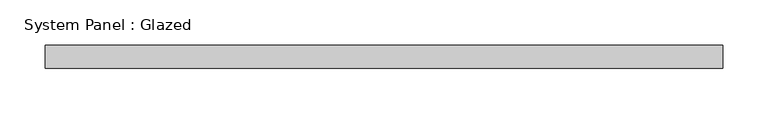
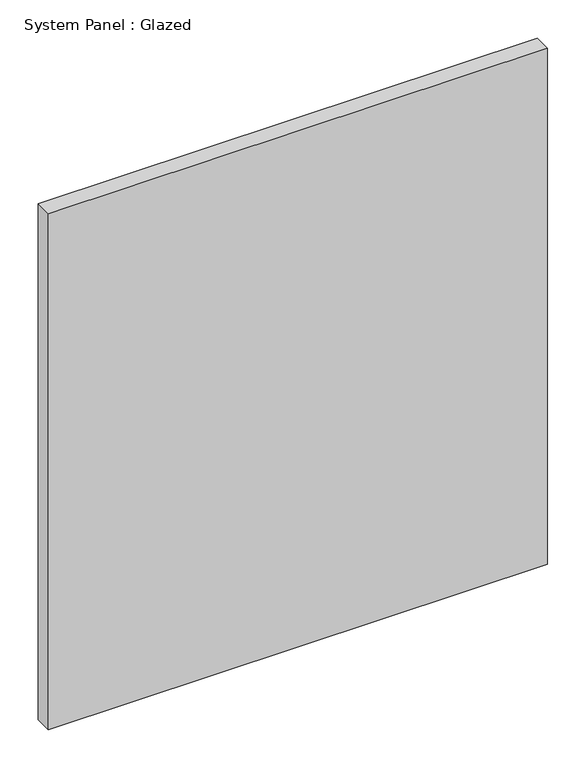
"""IFC4 building model written with IfcOpenShell, lengths in millimetres: plate geometry, System Panel : Glazed."""

from ifc_helpers import new_model, si_unit, origin, origin_with_axes, place, context, project, spatial, polyline, outline, extrude, source, transform, mapped, element, save


def system_panel_glazed_3c8ea7cb(model_context):
    return source(origin(), model_context, "Body", "SweptSolid", [
        extrude(outline(polyline([(374.65, 19.05), (-374.65, 19.05), (-374.65, 44.45), (374.65, 44.45), (374.65, 19.05)])), origin_with_axes(), (0.0, 0.0, 1.0), 818.549557),
    ])


if __name__ == "__main__":
    model = new_model("IFC4")
    model_context = context("Model", 3, world=origin())
    ifc_project = project(units=[si_unit("LENGTHUNIT", "METRE", prefix="MILLI")], contexts=[model_context])
    site = spatial("IfcSite", under=ifc_project)
    building = spatial("IfcBuilding", under=site)
    placement = place(None, origin())
    system_panel_glazed_shape = system_panel_glazed_3c8ea7cb(model_context)
    element("IfcPlate", 1, ObjectType="System Panel : Glazed", at=placement, inside=building, context=model_context, shape_type="MappedRepresentation", body=[
        mapped(system_panel_glazed_shape, transform((0.0, 0.0, 0.0), x_axis=(1.0, 0.0, 0.0), y_axis=(0.0, 1.0, 0.0), z_axis=(0.0, 0.0, 1.0))),
    ])
    save(model, "model.ifc")

# Revit data of these elements
# Type "System Panel : Glazed"
#   Construction Type Id = "GSP4R"
#   Analytic Construction = "1/8 in Pilkington single glazing"
#   Visual Light Transmittance = 0.9
#   Solar Heat Gain Coefficient = 0.86
#   Heat Transfer Coefficient (U) = 1.18115 BTU/(h·ft²·°F)
#   Define Thermal Properties by = 1
# Element 1 (IfcPlate, "System Panel : Glazed")
#   Materials on its faces: "Glass"
# Materials
#   "Glass": class "Glass", colour RGB 0 128 192, transparency 0.75, Description = "Soda Lime Glass", Cost = 0
